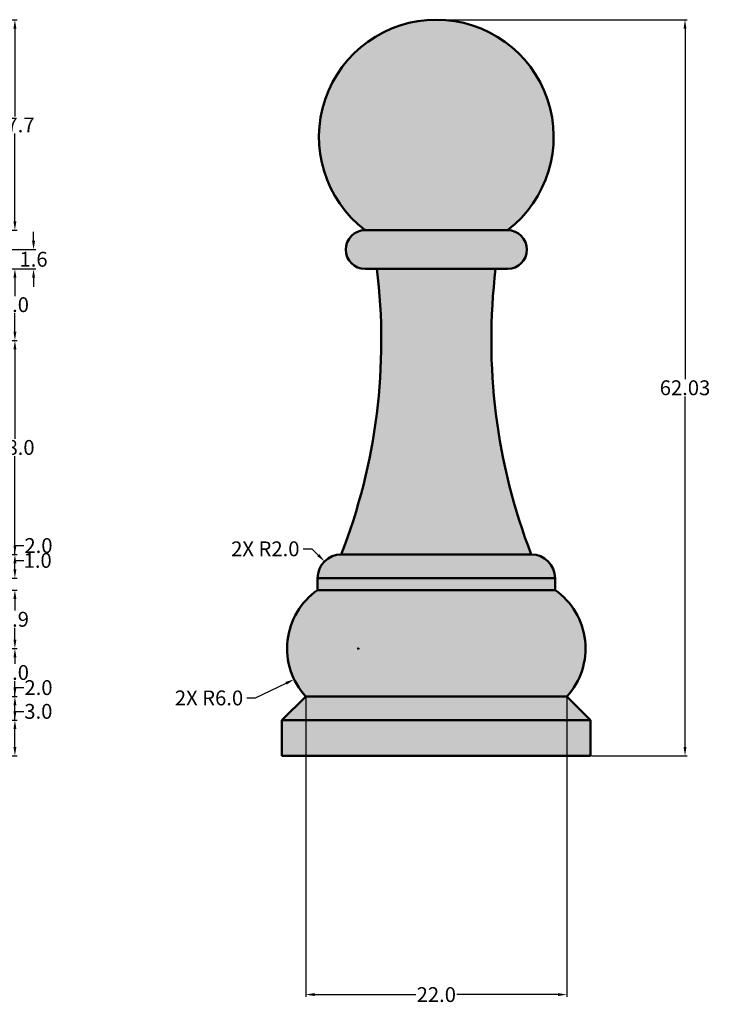
# Model space of a CAD drawing. Units: millimetres. Extents: x 10 to 184, y 6 to 153.
# Tile 2 of 2: x 125 to 184, y 6 to 89. Entities that reach past the tile are written whole.
import ezdxf

# ---------------------------------------------------------------- set-up
doc = ezdxf.new("R2010")
doc.units = ezdxf.units.MM
doc.header["$MEASUREMENT"] = 0
doc.layers.add('M-DIMS', color=2, linetype='Continuous', lineweight=25)
doc.layers.add('M-OUTL', color=7, linetype='Continuous', lineweight=50)
doc.layers.add('M-HATC', color=18, linetype='Continuous', lineweight=18, true_color=0x000000)
doc.styles.get("Standard").update_dxf_attribs({"font": 'arial.ttf'})
doc.dimstyles.get("Standard").update_dxf_attribs({"dimtxt": 1.25, "dimasz": 0.75, "dimexe": 0.18, "dimexo": 0.0625, "dimgap": 0.09, "dimtad": 0, "dimtih": 1, "dimtoh": 1, "dimdec": 1, "dimzin": 0, "dimdsep": 46, "dimtxsty": 'Standard', "dimcen": 0.09, "dimadec": 0, "dimazin": 0, "dimtfac": 1, "dimtdec": 1, "dimtofl": 0, "dimtmove": 0, "dimatfit": 3, "dimfxl": 1, "dimtolj": 1, "dimtzin": 0, "dimarcsym": 0})

# ---------------------------------------------------------------- blocks, each defined once
blk = doc.blocks.new('*D9')
at = {"layer": 'Defpoints', "color": 0, "transparency": 16777216}
for p in [(78.006, 29.562), (124.99, 29.562), (78.006, 26.562)]:
    blk.add_point(p, dxfattribs=at)
at = {"layer": 'M-DIMS', "color": 0, "lineweight": -2, "transparency": 16777216}
for p, q in [((124.99, 29.562), (124.99, 30.312)), ((124.99, 30.312), (125.74, 30.312)), ((78.068, 29.562), (125.17, 29.562)), ((124.99, 27.312), (124.99, 28.812)), ((78.068, 26.562), (125.17, 26.562))]:
    blk.add_line(p, q, dxfattribs=at)
at = {"layer": 'M-DIMS', "color": 0, "transparency": 16777216}
for points in [[(124.865, 28.812), (125.115, 28.812), (124.99, 29.562)], [(124.865, 27.312), (125.115, 27.312), (124.99, 26.562)]]:
    blk.add_solid(points, dxfattribs=at)
at = {"layer": 'M-DIMS', "color": 0, "transparency": 16777216, "insert": (126.965, 30.312), "char_height": 1.25, "attachment_point": 5}
blk.add_mtext('\\A1;3.0', dxfattribs=at)
blk = doc.blocks.new('*D10')
at = {"layer": 'Defpoints', "color": 0, "transparency": 16777216}
for p in [(76.006, 31.562), (124.99, 31.562), (78.006, 29.562)]:
    blk.add_point(p, dxfattribs=at)
at = {"layer": 'M-DIMS', "color": 0, "lineweight": -2, "transparency": 16777216}
for p, q in [((76.068, 31.562), (125.17, 31.562)), ((124.99, 31.562), (124.99, 32.312)), ((124.99, 32.312), (125.74, 32.312)), ((124.99, 30.312), (124.99, 30.812)), ((78.068, 29.562), (125.17, 29.562))]:
    blk.add_line(p, q, dxfattribs=at)
at = {"layer": 'M-DIMS', "color": 0, "transparency": 16777216}
for points in [[(124.865, 30.812), (125.115, 30.812), (124.99, 31.562)], [(124.865, 30.312), (125.115, 30.312), (124.99, 29.562)]]:
    blk.add_solid(points, dxfattribs=at)
at = {"layer": 'M-DIMS', "color": 0, "transparency": 16777216, "insert": (126.976, 32.312), "char_height": 1.25, "attachment_point": 5}
blk.add_mtext('\\A1;2.0', dxfattribs=at)
blk = doc.blocks.new('*D11')
at = {"layer": 'Defpoints', "color": 0, "transparency": 16777216}
for p in [(71.576, 35.609), (124.99, 35.609), (76.006, 31.562)]:
    blk.add_point(p, dxfattribs=at)
at = {"layer": 'M-DIMS', "color": 0, "lineweight": -2, "transparency": 16777216}
for p, q in [((71.638, 35.609), (125.17, 35.609)), ((124.99, 34.859), (124.99, 34.314)), ((124.99, 32.312), (124.99, 32.857)), ((76.068, 31.562), (125.17, 31.562))]:
    blk.add_line(p, q, dxfattribs=at)
at = {"layer": 'M-DIMS', "color": 0, "transparency": 16777216}
for points in [[(124.865, 34.859), (125.115, 34.859), (124.99, 35.609)], [(124.865, 32.312), (125.115, 32.312), (124.99, 31.562)]]:
    blk.add_solid(points, dxfattribs=at)
at = {"layer": 'M-DIMS', "color": 0, "transparency": 16777216, "insert": (124.99, 33.586), "char_height": 1.25, "attachment_point": 5}
blk.add_mtext('\\A1;4.0', dxfattribs=at)
blk = doc.blocks.new('*D12')
at = {"layer": 'Defpoints', "color": 0, "transparency": 16777216}
for p in [(75.006, 40.532), (124.99, 40.532), (71.576, 35.609)]:
    blk.add_point(p, dxfattribs=at)
at = {"layer": 'M-DIMS', "color": 0, "lineweight": -2, "transparency": 16777216}
for p, q in [((75.068, 40.532), (125.17, 40.532)), ((124.99, 39.782), (124.99, 38.799)), ((124.99, 36.359), (124.99, 37.342)), ((71.638, 35.609), (125.17, 35.609))]:
    blk.add_line(p, q, dxfattribs=at)
at = {"layer": 'M-DIMS', "color": 0, "transparency": 16777216}
for points in [[(124.865, 39.782), (125.115, 39.782), (124.99, 40.532)], [(124.865, 36.359), (125.115, 36.359), (124.99, 35.609)]]:
    blk.add_solid(points, dxfattribs=at)
at = {"layer": 'M-DIMS', "color": 0, "transparency": 16777216, "insert": (124.99, 38.071), "char_height": 1.25, "attachment_point": 5}
blk.add_mtext('\\A1;4.9', dxfattribs=at)
blk = doc.blocks.new('*D13')
at = {"layer": 'Defpoints', "color": 0, "transparency": 16777216}
for p in [(75.006, 41.532), (124.99, 41.532), (75.006, 40.532)]:
    blk.add_point(p, dxfattribs=at)
at = {"layer": 'M-DIMS', "color": 0, "lineweight": -2, "transparency": 16777216}
for p, q in [((124.99, 42.282), (124.99, 43.032)), ((124.99, 43.032), (125.74, 43.032)), ((75.068, 41.532), (125.17, 41.532)), ((75.068, 40.532), (125.17, 40.532)), ((124.99, 39.782), (124.99, 39.032))]:
    blk.add_line(p, q, dxfattribs=at)
at = {"layer": 'M-DIMS', "color": 0, "transparency": 16777216}
for points in [[(124.865, 42.282), (125.115, 42.282), (124.99, 41.532)], [(124.865, 39.782), (125.115, 39.782), (124.99, 40.532)]]:
    blk.add_solid(points, dxfattribs=at)
at = {"layer": 'M-DIMS', "color": 0, "transparency": 16777216, "insert": (126.906, 43.032), "char_height": 1.25, "attachment_point": 5}
blk.add_mtext('\\A1;1.0', dxfattribs=at)
blk = doc.blocks.new('*D14')
at = {"layer": 'Defpoints', "color": 0, "transparency": 16777216}
for p in [(73.006, 43.532), (124.99, 43.532), (75.006, 41.532)]:
    blk.add_point(p, dxfattribs=at)
at = {"layer": 'M-DIMS', "color": 0, "lineweight": -2, "transparency": 16777216}
for p, q in [((124.99, 43.532), (124.99, 44.282)), ((124.99, 44.282), (125.74, 44.282)), ((73.068, 43.532), (125.17, 43.532)), ((124.99, 42.282), (124.99, 42.782)), ((75.068, 41.532), (125.17, 41.532))]:
    blk.add_line(p, q, dxfattribs=at)
at = {"layer": 'M-DIMS', "color": 0, "transparency": 16777216}
for points in [[(124.865, 42.782), (125.115, 42.782), (124.99, 43.532)], [(124.865, 42.282), (125.115, 42.282), (124.99, 41.532)]]:
    blk.add_solid(points, dxfattribs=at)
at = {"layer": 'M-DIMS', "color": 0, "transparency": 16777216, "insert": (126.976, 44.282), "char_height": 1.25, "attachment_point": 5}
blk.add_mtext('\\A1;2.0', dxfattribs=at)
blk = doc.blocks.new('*D15')
at = {"layer": 'Defpoints', "color": 0, "transparency": 16777216}
for p in [(119.641, 61.564), (124.99, 61.564), (73.006, 43.532)]:
    blk.add_point(p, dxfattribs=at)
at = {"layer": 'M-DIMS', "color": 0, "lineweight": -2, "transparency": 16777216}
for p, q in [((119.703, 61.564), (125.17, 61.564)), ((124.99, 60.814), (124.99, 53.276)), ((124.99, 44.282), (124.99, 51.82)), ((73.068, 43.532), (125.17, 43.532))]:
    blk.add_line(p, q, dxfattribs=at)
at = {"layer": 'M-DIMS', "color": 0, "transparency": 16777216}
for points in [[(124.865, 60.814), (125.115, 60.814), (124.99, 61.564)], [(124.865, 44.282), (125.115, 44.282), (124.99, 43.532)]]:
    blk.add_solid(points, dxfattribs=at)
at = {"layer": 'M-DIMS', "color": 0, "transparency": 16777216, "insert": (124.99, 52.548), "char_height": 1.25, "attachment_point": 5}
blk.add_mtext('\\A1;18.0', dxfattribs=at)
blk = doc.blocks.new('*D16')
at = {"layer": 'Defpoints', "color": 0, "transparency": 16777216}
for p in [(71.006, 67.592), (124.99, 67.592), (119.641, 61.564)]:
    blk.add_point(p, dxfattribs=at)
at = {"layer": 'M-DIMS', "color": 0, "lineweight": -2, "transparency": 16777216}
for p, q in [((71.068, 67.592), (125.17, 67.592)), ((124.99, 66.842), (124.99, 65.306)), ((124.99, 62.314), (124.99, 63.85)), ((119.703, 61.564), (125.17, 61.564))]:
    blk.add_line(p, q, dxfattribs=at)
at = {"layer": 'M-DIMS', "color": 0, "transparency": 16777216}
for points in [[(124.865, 66.842), (125.115, 66.842), (124.99, 67.592)], [(124.865, 62.314), (125.115, 62.314), (124.99, 61.564)]]:
    blk.add_solid(points, dxfattribs=at)
at = {"layer": 'M-DIMS', "color": 0, "transparency": 16777216, "insert": (124.99, 64.578), "char_height": 1.25, "attachment_point": 5}
blk.add_mtext('\\A1;6.0', dxfattribs=at)
blk = doc.blocks.new('*D17')
at = {"layer": 'Defpoints', "color": 0, "transparency": 16777216}
for p in [(71.006, 69.222), (126.561, 69.222), (71.006, 67.592)]:
    blk.add_point(p, dxfattribs=at)
at = {"layer": 'M-DIMS', "color": 0, "lineweight": -2, "transparency": 16777216}
for p, q in [((126.561, 69.972), (126.561, 70.722)), ((71.068, 69.222), (126.741, 69.222)), ((71.068, 67.592), (126.741, 67.592)), ((126.561, 66.842), (126.561, 66.092))]:
    blk.add_line(p, q, dxfattribs=at)
at = {"layer": 'M-DIMS', "color": 0, "transparency": 16777216}
for points in [[(126.436, 69.972), (126.686, 69.972), (126.561, 69.222)], [(126.436, 66.842), (126.686, 66.842), (126.561, 67.592)]]:
    blk.add_solid(points, dxfattribs=at)
at = {"layer": 'M-DIMS', "color": 0, "transparency": 16777216, "insert": (126.561, 68.407), "char_height": 1.25, "attachment_point": 5}
blk.add_mtext('\\A1;1.6', dxfattribs=at)
blk = doc.blocks.new('*D19')
at = {"layer": 'Defpoints', "color": 0, "transparency": 16777216}
for p in [(65.006, 88.591), (124.99, 88.591), (71.006, 70.852)]:
    blk.add_point(p, dxfattribs=at)
at = {"layer": 'M-DIMS', "color": 0, "lineweight": -2, "transparency": 16777216}
for p, q in [((65.068, 88.591), (125.17, 88.591)), ((124.99, 87.841), (124.99, 80.439)), ((124.99, 71.602), (124.99, 79.004)), ((71.068, 70.852), (125.17, 70.852))]:
    blk.add_line(p, q, dxfattribs=at)
at = {"layer": 'M-DIMS', "color": 0, "transparency": 16777216}
for points in [[(124.865, 87.841), (125.115, 87.841), (124.99, 88.591)], [(124.865, 71.602), (125.115, 71.602), (124.99, 70.852)]]:
    blk.add_solid(points, dxfattribs=at)
at = {"layer": 'M-DIMS', "color": 0, "transparency": 16777216, "insert": (124.99, 79.722), "char_height": 1.25, "attachment_point": 5}
blk.add_mtext('\\A1;17.7', dxfattribs=at)
blk = doc.blocks.new('PAWN-ELEVATION')
for p, q in [((13, 44.29), (7, 44.29)), ((13, 44.29), (19, 44.29)), ((13, 41.03), (7, 41.03)), ((13, 41.03), (8, 41.03)), ((13, 41.03), (19, 41.03)), ((5, 16.97), (21, 16.97)), ((3, 13.97), (3, 14.97)), ((3, 14.97), (23, 14.97)), ((23, 14.97), (23, 13.97)), ((3, 13.97), (23, 13.97)), ((0, 3), (2, 5)), ((2, 5), (24, 5)), ((26, 3), (24, 5)), ((26, 3), (0, 3)), ((0, 3), (0, 0)), ((26, 0), (26, 3)), ((0, 0), (26, 0))]:
    blk.add_line(p, q)
for centre, radius, start, end in [((13, 52.145), 9.884, 307.37421, 232.62579), ((7, 42.66), 1.63, 90, 270), ((19, 42.66), 1.63, 270, 90), ((-41.636, 35.002), 50, 338.86061, 6.92453), ((67.635, 35.002), 50, 173.07547, 201.13939), ((5, 14.97), 2, 90, 180), ((21, 14.97), 2, 360, 90), ((6.429, 9.047), 6, 124.86349, 222.41407), ((19.57, 9.047), 6, 317.58593, 55.13651)]:
    blk.add_arc(centre, radius, start, end)
blk = doc.blocks.new('*D31')
at = {"layer": 'Defpoints', "color": 0, "transparency": 16777216}
for p in [(160.486, 88.591), (181.436, 88.591), (173.486, 26.562)]:
    blk.add_point(p, dxfattribs=at)
at = {"layer": 'M-DIMS', "color": 0, "lineweight": -2, "transparency": 16777216}
for p, q in [((160.549, 88.591), (181.616, 88.591)), ((181.436, 87.841), (181.436, 58.305)), ((181.436, 27.312), (181.436, 56.848)), ((173.549, 26.562), (181.616, 26.562))]:
    blk.add_line(p, q, dxfattribs=at)
at = {"layer": 'M-DIMS', "color": 0, "transparency": 16777216}
for points in [[(181.311, 87.841), (181.561, 87.841), (181.436, 88.591)], [(181.311, 27.312), (181.561, 27.312), (181.436, 26.562)]]:
    blk.add_solid(points, dxfattribs=at)
at = {"layer": 'M-DIMS', "color": 0, "transparency": 16777216, "insert": (181.436, 57.577), "char_height": 1.25, "attachment_point": 5}
blk.add_mtext('\\A1;62.03', dxfattribs=at)
blk = doc.blocks.new('*D32')
at = {"layer": 'Defpoints', "color": 0, "transparency": 16777216}
for p in [(149.486, 31.562), (171.486, 31.562), (171.486, 6.447)]:
    blk.add_point(p, dxfattribs=at)
at = {"layer": 'M-DIMS', "color": 0, "lineweight": -2, "transparency": 16777216}
for p, q in [((149.486, 31.5), (149.486, 6.267)), ((171.486, 31.5), (171.486, 6.267)), ((150.236, 6.447), (158.764, 6.447)), ((170.736, 6.447), (162.208, 6.447))]:
    blk.add_line(p, q, dxfattribs=at)
at = {"layer": 'M-DIMS', "color": 0, "transparency": 16777216}
for points in [[(150.236, 6.572), (150.236, 6.322), (149.486, 6.447)], [(170.736, 6.572), (170.736, 6.322), (171.486, 6.447)]]:
    blk.add_solid(points, dxfattribs=at)
at = {"layer": 'M-DIMS', "color": 0, "transparency": 16777216, "insert": (160.486, 6.447), "char_height": 1.25, "attachment_point": 5}
blk.add_mtext('\\A1;22.0', dxfattribs=at)
blk = doc.blocks.new('*D38')
at = {"layer": 'Defpoints', "color": 0, "transparency": 16777216}
for p in [(153.916, 35.609), (148.511, 33.005)]:
    blk.add_point(p, dxfattribs=at)
at = {"layer": 'M-DIMS', "color": 0, "lineweight": -2, "transparency": 16777216}
for p, q in [((153.916, 35.519), (153.916, 35.699)), ((153.826, 35.609), (154.006, 35.609)), ((145.267, 31.443), (147.835, 32.68)), ((144.517, 31.443), (145.267, 31.443))]:
    blk.add_line(p, q, dxfattribs=at)
at = {"layer": 'M-DIMS', "color": 0, "transparency": 16777216}
blk.add_solid([(147.781, 32.792), (147.889, 32.567), (148.511, 33.005)], dxfattribs=at)
at = {"layer": 'M-DIMS', "color": 0, "transparency": 16777216, "insert": (141.34, 31.443), "char_height": 1.25, "attachment_point": 5}
blk.add_mtext('\\A1;2X R6.0', dxfattribs=at)
blk = doc.blocks.new('*D39')
at = {"layer": 'Defpoints', "color": 0, "transparency": 16777216}
for p in [(151.072, 42.946), (152.486, 41.532)]:
    blk.add_point(p, dxfattribs=at)
at = {"layer": 'M-DIMS', "color": 0, "lineweight": -2, "transparency": 16777216}
for p, q in [((149.261, 44.006), (150.011, 44.006)), ((150.011, 44.006), (150.542, 43.476)), ((152.396, 41.532), (152.576, 41.532)), ((152.486, 41.442), (152.486, 41.622))]:
    blk.add_line(p, q, dxfattribs=at)
at = {"layer": 'M-DIMS', "color": 0, "transparency": 16777216}
blk.add_solid([(150.63, 43.565), (150.453, 43.388), (151.072, 42.946)], dxfattribs=at)
at = {"layer": 'M-DIMS', "color": 0, "transparency": 16777216, "insert": (146.084, 44.006), "char_height": 1.25, "attachment_point": 5}
blk.add_mtext('\\A1;2X R2.0', dxfattribs=at)

msp = doc.modelspace()

# ---------------------------------------------------------------- hatches: boundary and pattern name
at = {"layer": 'M-HATC'}
h = msp.add_hatch(color=256, dxfattribs=at)
h.dxf.hatch_style = 1
h.paths.add_polyline_path([(154.4865, 70.8521), (160.4865, 70.8521), (166.4865, 70.8521, 2.9565638)])
h.paths.add_polyline_path([(165.4865, 67.5921), (160.4865, 67.5921), (155.4865, 67.5921, -0.1230677), (152.4865, 43.5321), (168.4865, 43.5321, -0.1230677)])
h.paths.add_polyline_path([(170.4865, 40.5321), (150.4865, 40.5321, 0.4533601), (149.4865, 31.5621), (171.4865, 31.5621, 0.4533601)])
h.paths.add_polyline_path([(166.4865, 70.8521), (160.4865, 70.8521), (154.4865, 70.8521, 1), (154.4865, 67.5921), (160.4865, 67.5921), (165.4865, 67.5921), (166.4865, 67.5921, 1)])
h.paths.add_polyline_path([(170.4865, 41.5321), (150.4865, 41.5321), (150.4865, 40.5321), (170.4865, 40.5321)])
h.paths.add_polyline_path([(168.4865, 43.5321), (152.4865, 43.5321, 0.4142136), (150.4865, 41.5321), (170.4865, 41.5321, 0.4142136)])
h.paths.add_polyline_path([(171.4865, 31.5621), (149.4865, 31.5621), (147.4865, 29.5621), (173.4865, 29.5621)])
h.paths.add_polyline_path([(173.4865, 29.5621), (147.4865, 29.5621), (147.4865, 26.5621), (173.4865, 26.5621)])

# ---------------------------------------------------------------- block references
at = {"layer": 'M-OUTL'}
msp.add_blockref('PAWN-ELEVATION', (147.4869, 26.562), dxfattribs=at)

# ---------------------------------------------------------------- dimensions: what is measured, and where the dimension line sits
at = {"layer": 'M-DIMS'}
for base, p1, p2, angle, override, picture, middle in [((124.9896, 88.5914), (71.0055, 70.8521), (65.0055, 88.5914), 270, {"dimclrd": 0, "dimclre": 0, "dimclrt": 0}, '*D19', (124.9896, 79.7218)), ((181.4365, 88.5914), (173.4865, 26.5621), (160.4865, 88.5914), 90, {"dimdec": 2, "dimlfac": 1, "dimrnd": 0, "dimzin": 0, "dimdsep": 46, "dimlunit": 2}, '*D31', (181.4365, 57.5768)), ((124.9896, 67.5921), (119.6408, 61.564), (71.0055, 67.5921), 270, {"dimclrd": 0, "dimclre": 0, "dimclrt": 0}, '*D16', (124.9896, 64.578)), ((124.9896, 61.564), (73.0055, 43.5321), (119.6408, 61.564), 270, {"dimclrd": 0, "dimclre": 0, "dimclrt": 0}, '*D15', (124.9896, 52.548)), ((124.9896, 43.5321), (75.0055, 41.5321), (73.0055, 43.5321), 270, {"dimclrd": 0, "dimclre": 0, "dimclrt": 0}, '*D14', (126.976, 44.2821)), ((124.9896, 41.5321), (75.0055, 40.5321), (75.0055, 41.5321), 270, {"dimclrd": 0, "dimclre": 0, "dimclrt": 0}, '*D13', (126.9065, 43.0321)), ((124.9896, 40.5321), (71.5758, 35.609), (75.0055, 40.5321), 270, {"dimclrd": 0, "dimclre": 0, "dimclrt": 0}, '*D12', (124.9896, 38.0705)), ((124.9896, 35.609), (76.0055, 31.5621), (71.5758, 35.609), 270, {"dimclrd": 0, "dimclre": 0, "dimclrt": 0}, '*D11', (124.9896, 33.5855)), ((124.9896, 31.5621), (78.0055, 29.5621), (76.0055, 31.5621), 270, {"dimclrd": 0, "dimclre": 0, "dimclrt": 0}, '*D10', (126.976, 32.3121)), ((124.9896, 29.5621), (78.0055, 26.5621), (78.0055, 29.5621), 270, {"dimclrd": 0, "dimclre": 0, "dimclrt": 0}, '*D9', (126.9649, 30.3121))]:
    dim = msp.add_linear_dim(base=base, p1=p1, p2=p2, angle=angle, dimstyle='Standard', override=override, dxfattribs=at)
    dim.commit()
    dim.dimension.update_dxf_attribs({"geometry": picture, "text_midpoint": middle})
dim = msp.add_linear_dim(base=(126.561, 69.2221), p1=(71.0055, 67.5921), p2=(71.0055, 69.2221), angle=270, dimstyle='Standard', override={"dimclrd": 0, "dimclre": 0, "dimclrt": 0}, dxfattribs=at)
dim.commit()
dim.dimension.update_dxf_attribs({"geometry": '*D17', "text_midpoint": (126.561, 68.4071), "dimtype": 160})
dim = msp.add_radius_dim(center=(152.4865, 41.5321), mpoint=(151.072, 42.946), text='2X <>', dimstyle='Standard', override={"dimdec": 1, "dimlfac": 1, "dimrnd": 0, "dimzin": 0, "dimdsep": 46, "dimlunit": 2}, dxfattribs=at)
dim.commit()
dim.dimension.update_dxf_attribs({"geometry": '*D39', "text_midpoint": (146.0836, 44.0065)})
dim = msp.add_radius_dim(center=(153.9162, 35.609), mpoint=(148.5107, 33.0051), text='2X <>', dimstyle='Standard', override={"dimdec": 1, "dimlfac": 1, "dimrnd": 0, "dimzin": 0, "dimdsep": 46, "dimlunit": 2}, dxfattribs=at)
dim.commit()
dim.dimension.update_dxf_attribs({"geometry": '*D38', "text_midpoint": (141.3398, 31.4428), "dimtype": 164})
dim = msp.add_linear_dim(base=(171.4865, 6.4471), p1=(149.4865, 31.5621), p2=(171.4865, 31.5621), dimstyle='Standard', override={"dimdec": 1, "dimlfac": 1, "dimrnd": 0, "dimzin": 0, "dimdsep": 46, "dimlunit": 2}, dxfattribs=at)
dim.commit()
dim.dimension.update_dxf_attribs({"geometry": '*D32', "text_midpoint": (160.4865, 6.4471)})

doc.saveas('drawing.dxf')
